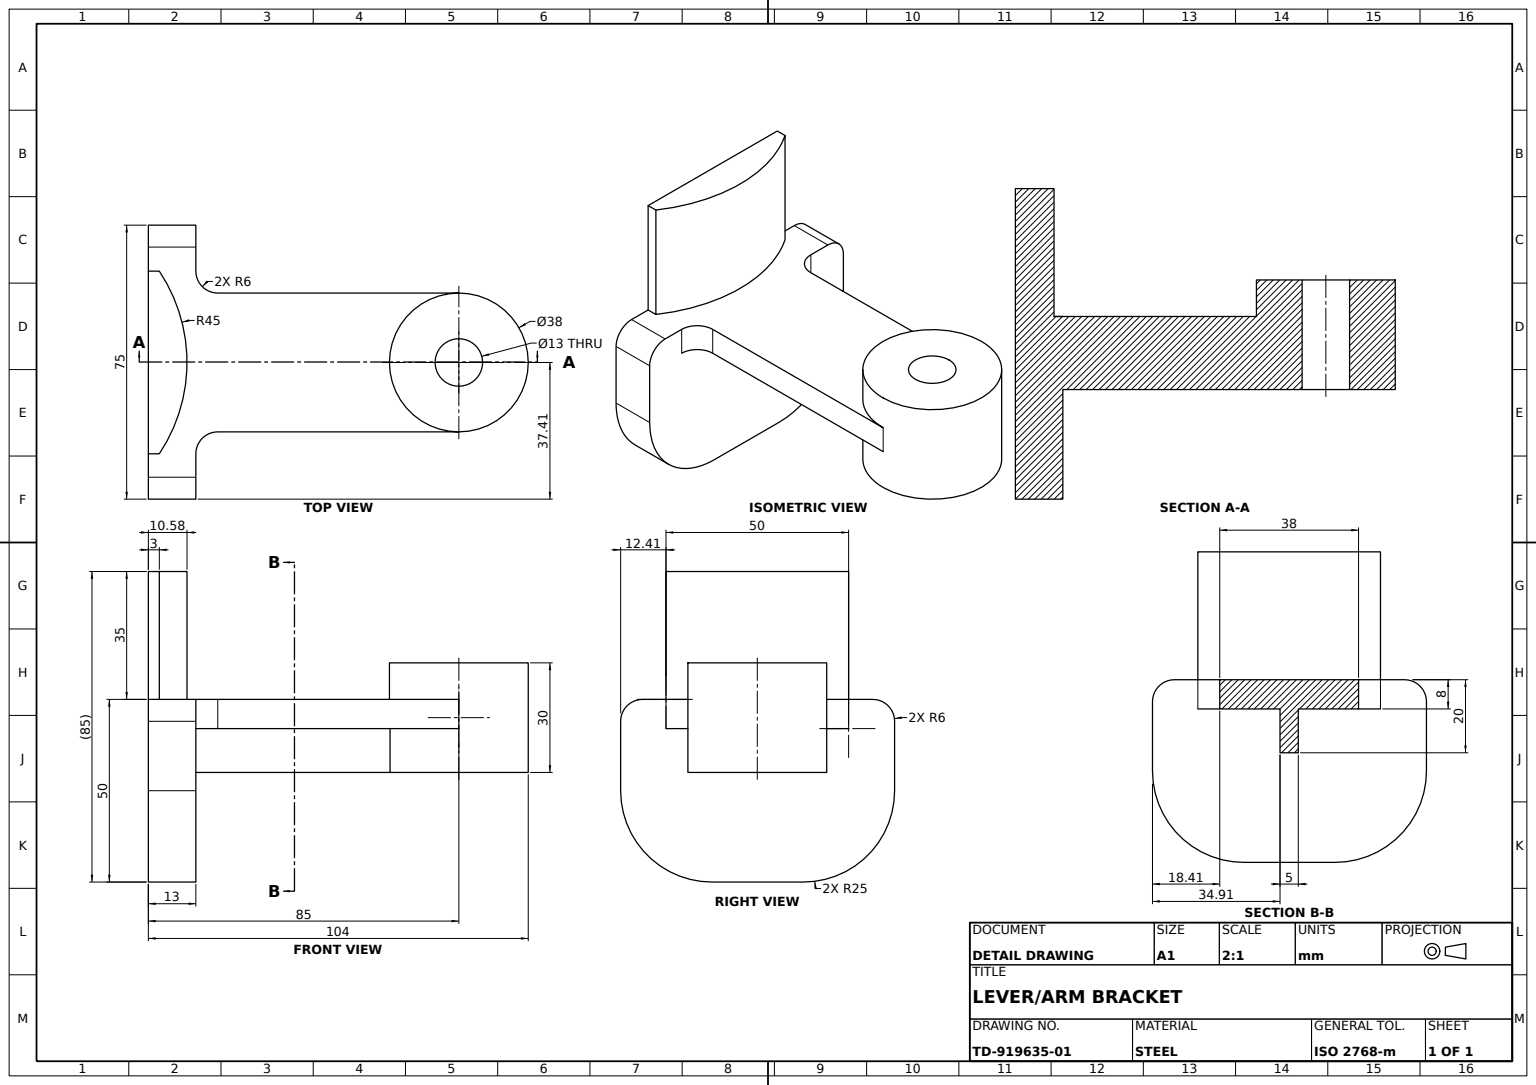
from build123d import *

# Parameters (mm, degrees)
BASE_BLOCK_SKETCH_W   = 13
BASE_BLOCK_SKETCH_H   = 50
BASE_BLOCK_DEPTH      = 75
BASE_END_ROUND_R25_R  = 25
BASE_EDGE_FILLET_R6_R = 6
ARM_WEB_DEPTH         = 35
HUB_BOSS_SKETCH_R     = 19
HUB_BOSS_SKETCH_R_2   = 6.5
HUB_BOSS_DEPTH        = 30
UPPER_LUG_DEPTH       = 8
CURVED_START          = -20
CURVED_BLADE_DEPTH    = 20
LUG_FILLET_R6_A_R     = 6
LUG_FILLET_R6_B_R     = 6


with BuildPart() as part:
    # Base Block Sketch → Base Block (new body)
    with BuildSketch(Plane.XY):
        with Locations((6.5, 25)):
            Rectangle(BASE_BLOCK_SKETCH_W, BASE_BLOCK_SKETCH_H)
    extrude(amount=-BASE_BLOCK_DEPTH)

    # Base End Round R25
    base_end_round_r25_edges = [part.edges().sort_by_distance(p)[0] for p in [
        (6.5, 0, 0),
        (6.5, 0, -75),
    ]]
    fillet(base_end_round_r25_edges, radius=BASE_END_ROUND_R25_R)

    # Base Edge Fillet R6
    base_edge_fillet_r6_edges = [part.edges().sort_by_distance(p)[0] for p in [
        (6.5, 50, -75),
        (6.5, 50, 0),
    ]]
    fillet(base_edge_fillet_r6_edges, radius=BASE_EDGE_FILLET_R6_R)

    # Arm Web Sketch → Arm Web (add)
    with BuildSketch(Plane(origin=(0, 50, 0), x_dir=(1, 0, 0), z_dir=(0, 1, 0))):
        with BuildLine():
            Line((3, 62.41287987), (0, 62.41287987))
            Line((0, 62.41287987), (0, 37.41287987))
            Line((0, 37.41287987), (0, 12.41287987))
            Line((0, 12.41287987), (3, 12.41287987))
            ThreePointArc((3, 12.41287987), (10.583426132, 37.41287987), (3, 62.41287987))
        make_face()
    extrude(amount=ARM_WEB_DEPTH)



with BuildPart() as body_2:
    # Hub Boss Sketch → Hub Boss (new body)
    with BuildSketch(Plane(origin=(0, 30, 0), x_dir=(1, 0, 0), z_dir=(0, 1, 0))):
        with Locations(Location((85, 37.41287987, 0), (0, 0, 270))):
            Circle(HUB_BOSS_SKETCH_R)
        with Locations(Location((85, 37.41287987, 0), (0, 0, 270))):
            Circle(HUB_BOSS_SKETCH_R_2, mode=Mode.SUBTRACT)
    extrude(amount=HUB_BOSS_DEPTH)


with BuildPart() as part_1:
    add(part.part)

    add(body_2.part)  # Upper Lug merges body 2
    # Upper Lug Sketch → Upper Lug (add)
    with BuildSketch(Plane(origin=(0, 50, 0), x_dir=(1, 0, 0), z_dir=(0, 1, 0))):
        with BuildLine():
            Line((85, 56.41287987), (13, 56.41287987))
            Line((13, 56.41287987), (13, 18.41287987))
            Line((13, 18.41287987), (85, 18.41287987))
            ThreePointArc((85, 18.41287987), (66, 37.41287987), (85, 56.41287987))
        make_face()
    extrude(amount=-UPPER_LUG_DEPTH)

    # Curved Blade Sketch → Curved Blade (add)
    with BuildSketch(Plane(origin=(0, 50, 0), x_dir=(1, 0, 0), z_dir=(0, 1, 0)).offset(CURVED_START)):
        with BuildLine():
            Line((0, 34.91287987), (66.165191798, 34.91287987))
            ThreePointArc((66.165191798, 34.91287987), (66, 37.41287987), (66.165191798, 39.91287987))
            Line((66.165191798, 39.91287987), (0, 39.91287987))
            Line((0, 39.91287987), (0, 34.91287987))
        make_face()
    extrude(amount=CURVED_BLADE_DEPTH)

    # Lug Fillet R6 A
    lug_fillet_r6_a_edges = [part_1.edges().sort_by_distance(p)[0] for p in [
        (13, 46, -18.41287987),
    ]]
    fillet(lug_fillet_r6_a_edges, radius=LUG_FILLET_R6_A_R)

    # Lug Fillet R6 B
    lug_fillet_r6_b_edges = [part_1.edges().sort_by_distance(p)[0] for p in [
        (13, 46, -56.41287987),
    ]]
    fillet(lug_fillet_r6_b_edges, radius=LUG_FILLET_R6_B_R)


solid = part_1.part
